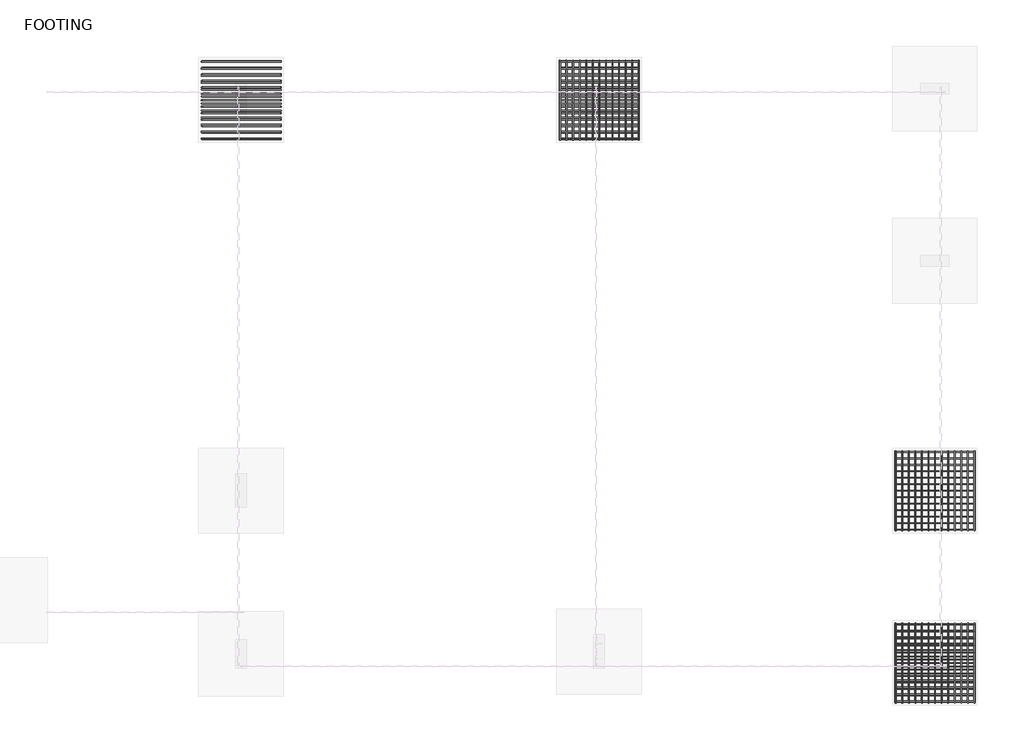
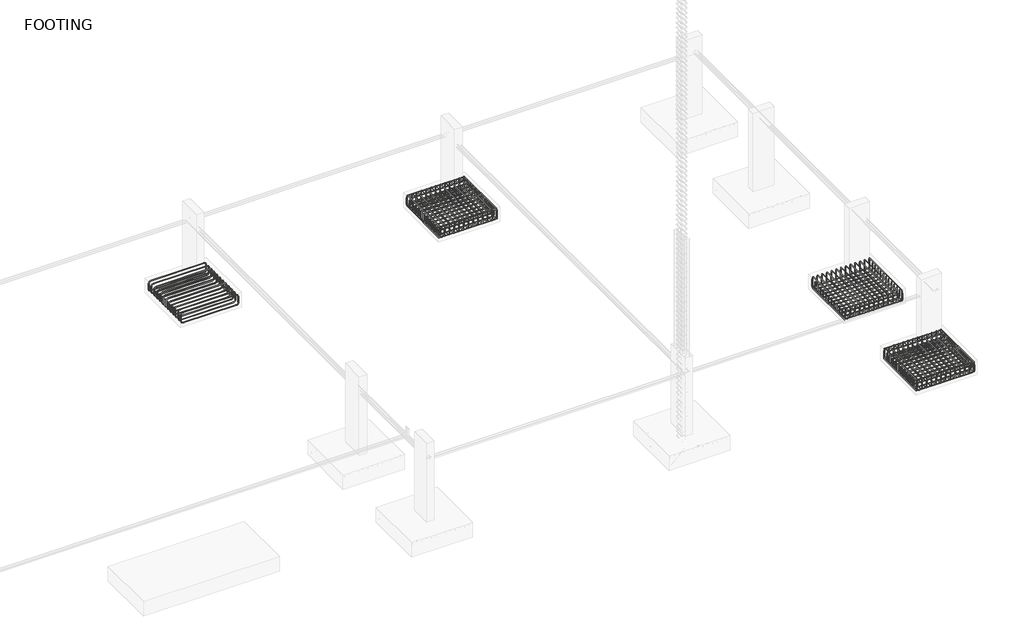
# One storey, part 8 of 12: 13 reinforcing bars.
"""IFC4 building model written with IfcOpenShell, lengths in millimetres."""

from ifc_helpers import new_model, si_unit, point, frame, origin, place, context, project, spatial, polyline, circle_curve, trimmed, segment, composite_curve, source, transform, mapped, element, save
from ifc_brep_helpers import swept_disk

model = new_model("IFC4")

# Units and contexts
model_context = context("Model", 3, world=origin())
ifc_project = project(units=[si_unit("LENGTHUNIT", "METRE", prefix="MILLI")], contexts=[model_context])

# Site, building, storey
site = spatial("IfcSite", under=ifc_project)
building = spatial("IfcBuilding", under=site)
storey = spatial("IfcBuildingStorey", under=building, Name="FOOTING", Elevation=-5638.8)

# Reinforcing bars
placement = place(None, origin())
reinforcing_bar_shape = source(origin(), model_context, "Body", "SolidModel", [
    swept_disk(composite_curve([segment(polyline([(20052.0998335, -15200.9541655, -5788.8), (20052.0998335, -15200.9541655, -5975.4)]), True, "CONTINUOUS"), segment(trimmed(circle_curve(frame((20052.0998335, -15145.5041655, -5975.4), z_axis=(1.0, 0.0, 0.0), x_axis=(0.0, -55.44999999999891, 0.0)), 55.45), [point((20052.0998335, -15200.9541655, -5975.4))], [point((20052.0998335, -15145.5041655, -6030.85))], True, "CARTESIAN"), True, "CONTINUOUS"), segment(polyline([(20052.0998335, -15145.5041655, -6030.85), (20052.0998335, -13572.3041655, -6030.85)]), True, "CONTINUOUS"), segment(trimmed(circle_curve(frame((20052.0998335, -13572.3041655, -5975.4), z_axis=(1.0, 0.0, 0.0), x_axis=(0.0, 0.0, -55.45000000000073)), 55.45), [point((20052.0998335, -13572.3041655, -6030.85))], [point((20052.0998335, -13516.8541655, -5975.4))], True, "CARTESIAN"), True, "CONTINUOUS"), segment(polyline([(20052.0998335, -13516.8541655, -5975.4), (20052.0998335, -13516.8541655, -5788.8)]), True, "CONTINUOUS")], self_intersect=False), 7.95),
])
element("IfcReinforcingBar", 1, at=placement, inside=storey, context=model_context, shape_type="MappedRepresentation", body=[
    mapped(reinforcing_bar_shape, transform((0.0, 0.0, 0.0), x_axis=(1.0, 0.0, 0.0), y_axis=(0.0, 1.0, 0.0), z_axis=(0.0, 0.0, 1.0))),
    mapped(reinforcing_bar_shape, transform((-140.3416667, 0.0, 0.0), x_axis=(1.0, 0.0, 0.0), y_axis=(0.0, 1.0, 0.0), z_axis=(0.0, 0.0, 1.0))),
    mapped(reinforcing_bar_shape, transform((-280.6833333, 0.0, 0.0), x_axis=(1.0, 0.0, 0.0), y_axis=(0.0, 1.0, 0.0), z_axis=(0.0, 0.0, 1.0))),
    mapped(reinforcing_bar_shape, transform((-421.025, 0.0, 0.0), x_axis=(1.0, 0.0, 0.0), y_axis=(0.0, 1.0, 0.0), z_axis=(0.0, 0.0, 1.0))),
    mapped(reinforcing_bar_shape, transform((-561.3666667, 0.0, 0.0), x_axis=(1.0, 0.0, 0.0), y_axis=(0.0, 1.0, 0.0), z_axis=(0.0, 0.0, 1.0))),
    mapped(reinforcing_bar_shape, transform((-701.7083333, 0.0, 0.0), x_axis=(1.0, 0.0, 0.0), y_axis=(0.0, 1.0, 0.0), z_axis=(0.0, 0.0, 1.0))),
    mapped(reinforcing_bar_shape, transform((-842.05, 0.0, 0.0), x_axis=(1.0, 0.0, 0.0), y_axis=(0.0, 1.0, 0.0), z_axis=(0.0, 0.0, 1.0))),
    mapped(reinforcing_bar_shape, transform((-982.3916667, 0.0, 0.0), x_axis=(1.0, 0.0, 0.0), y_axis=(0.0, 1.0, 0.0), z_axis=(0.0, 0.0, 1.0))),
    mapped(reinforcing_bar_shape, transform((-1122.7333333, 0.0, 0.0), x_axis=(1.0, 0.0, 0.0), y_axis=(0.0, 1.0, 0.0), z_axis=(0.0, 0.0, 1.0))),
    mapped(reinforcing_bar_shape, transform((-1263.075, 0.0, 0.0), x_axis=(1.0, 0.0, 0.0), y_axis=(0.0, 1.0, 0.0), z_axis=(0.0, 0.0, 1.0))),
    mapped(reinforcing_bar_shape, transform((-1403.4166667, 0.0, 0.0), x_axis=(1.0, 0.0, 0.0), y_axis=(0.0, 1.0, 0.0), z_axis=(0.0, 0.0, 1.0))),
    mapped(reinforcing_bar_shape, transform((-1543.7583333, 0.0, 0.0), x_axis=(1.0, 0.0, 0.0), y_axis=(0.0, 1.0, 0.0), z_axis=(0.0, 0.0, 1.0))),
    mapped(reinforcing_bar_shape, transform((-1684.1, 0.0, 0.0), x_axis=(1.0, 0.0, 0.0), y_axis=(0.0, 1.0, 0.0), z_axis=(0.0, 0.0, 1.0))),
])
reinforcing_bar_2_shape = source(origin(), model_context, "Body", "SolidModel", [
    swept_disk(composite_curve([segment(polyline([(20042.9597994, -13515.2541655, -5888.8), (20042.9597994, -13515.2541655, -5741.5)]), True, "CONTINUOUS"), segment(trimmed(circle_curve(frame((20042.9597994, -13561.6041655, -5741.5), z_axis=(1.0, 0.0, 0.0), x_axis=(0.0, 46.350000000000364, 0.0)), 46.35), [point((20042.9597994, -13515.2541655, -5741.5))], [point((20042.9597994, -13561.6041655, -5695.15))], True, "CARTESIAN"), True, "CONTINUOUS"), segment(polyline([(20042.9597994, -13561.6041655, -5695.15), (20042.9597994, -15156.2041655, -5695.15)]), True, "CONTINUOUS"), segment(trimmed(circle_curve(frame((20042.9597994, -15156.2041655, -5741.5), z_axis=(1.0, 0.0, 0.0), x_axis=(0.0, 0.0, 46.350000000000364)), 46.35), [point((20042.9597994, -15156.2041655, -5695.15))], [point((20042.9597994, -15202.5541655, -5741.5))], True, "CARTESIAN"), True, "CONTINUOUS"), segment(polyline([(20042.9597994, -15202.5541655, -5741.5), (20042.9597994, -15202.5541655, -5888.8)]), True, "CONTINUOUS")], self_intersect=False), 6.35),
])
element("IfcReinforcingBar", 2, at=placement, inside=storey, context=model_context, shape_type="MappedRepresentation", body=[
    mapped(reinforcing_bar_2_shape, transform((0.0, 0.0, 0.0), x_axis=(1.0, 0.0, 0.0), y_axis=(0.0, 1.0, 0.0), z_axis=(0.0, 0.0, 1.0))),
    mapped(reinforcing_bar_2_shape, transform((-138.4829293, 0.0, 0.0), x_axis=(1.0, 0.0, 0.0), y_axis=(0.0, 1.0, 0.0), z_axis=(0.0, 0.0, 1.0))),
    mapped(reinforcing_bar_2_shape, transform((-276.9658586, 0.0, 0.0), x_axis=(1.0, 0.0, 0.0), y_axis=(0.0, 1.0, 0.0), z_axis=(0.0, 0.0, 1.0))),
    mapped(reinforcing_bar_2_shape, transform((-415.4487879, 0.0, 0.0), x_axis=(1.0, 0.0, 0.0), y_axis=(0.0, 1.0, 0.0), z_axis=(0.0, 0.0, 1.0))),
    mapped(reinforcing_bar_2_shape, transform((-553.9317172, 0.0, 0.0), x_axis=(1.0, 0.0, 0.0), y_axis=(0.0, 1.0, 0.0), z_axis=(0.0, 0.0, 1.0))),
    mapped(reinforcing_bar_2_shape, transform((-692.4146465, 0.0, 0.0), x_axis=(1.0, 0.0, 0.0), y_axis=(0.0, 1.0, 0.0), z_axis=(0.0, 0.0, 1.0))),
    mapped(reinforcing_bar_2_shape, transform((-830.8975758, 0.0, 0.0), x_axis=(1.0, 0.0, 0.0), y_axis=(0.0, 1.0, 0.0), z_axis=(0.0, 0.0, 1.0))),
    mapped(reinforcing_bar_2_shape, transform((-969.3805051, 0.0, 0.0), x_axis=(1.0, 0.0, 0.0), y_axis=(0.0, 1.0, 0.0), z_axis=(0.0, 0.0, 1.0))),
    mapped(reinforcing_bar_2_shape, transform((-1107.8634344, 0.0, 0.0), x_axis=(1.0, 0.0, 0.0), y_axis=(0.0, 1.0, 0.0), z_axis=(0.0, 0.0, 1.0))),
    mapped(reinforcing_bar_2_shape, transform((-1246.3463637, 0.0, 0.0), x_axis=(1.0, 0.0, 0.0), y_axis=(0.0, 1.0, 0.0), z_axis=(0.0, 0.0, 1.0))),
    mapped(reinforcing_bar_2_shape, transform((-1384.8292929, 0.0, 0.0), x_axis=(1.0, 0.0, 0.0), y_axis=(0.0, 1.0, 0.0), z_axis=(0.0, 0.0, 1.0))),
    mapped(reinforcing_bar_2_shape, transform((-1523.3122222, 0.0, 0.0), x_axis=(1.0, 0.0, 0.0), y_axis=(0.0, 1.0, 0.0), z_axis=(0.0, 0.0, 1.0))),
    mapped(reinforcing_bar_2_shape, transform((-1661.7951515, 0.0, 0.0), x_axis=(1.0, 0.0, 0.0), y_axis=(0.0, 1.0, 0.0), z_axis=(0.0, 0.0, 1.0))),
])
reinforcing_bar_3_shape = source(origin(), model_context, "Body", "SolidModel", [
    swept_disk(composite_curve([segment(polyline([(18367.9998335, -15183.9041655, -5773.0), (18367.9998335, -15183.9041655, -5959.6)]), True, "CONTINUOUS"), segment(trimmed(circle_curve(frame((18423.4498335, -15183.9041655, -5959.6), z_axis=(0.0, -1.0, 0.0), x_axis=(-55.45000000000073, 0.0, 0.0)), 55.45), [point((18367.9998335, -15183.9041655, -5959.6))], [point((18423.4498335, -15183.9041655, -6015.05))], True, "CARTESIAN"), True, "CONTINUOUS"), segment(polyline([(18423.4498335, -15183.9041655, -6015.05), (19996.6498335, -15183.9041655, -6015.05)]), True, "CONTINUOUS"), segment(trimmed(circle_curve(frame((19996.6498335, -15183.9041655, -5959.6), z_axis=(0.0, -1.0, 0.0), x_axis=(0.0, 0.0, -55.44999999999982)), 55.45), [point((19996.6498335, -15183.9041655, -6015.05))], [point((20052.0998335, -15183.9041655, -5959.6))], True, "CARTESIAN"), True, "CONTINUOUS"), segment(polyline([(20052.0998335, -15183.9041655, -5959.6), (20052.0998335, -15183.9041655, -5773.0)]), True, "CONTINUOUS")], self_intersect=False), 7.95),
])
element("IfcReinforcingBar", 3, at=placement, inside=storey, context=model_context, shape_type="MappedRepresentation", body=[
    mapped(reinforcing_bar_3_shape, transform((0.0, 0.0, 0.0), x_axis=(1.0, 0.0, 0.0), y_axis=(0.0, 1.0, 0.0), z_axis=(0.0, 0.0, 1.0))),
    mapped(reinforcing_bar_3_shape, transform((0.0, 137.7402087, 0.0), x_axis=(1.0, 0.0, 0.0), y_axis=(0.0, 1.0, 0.0), z_axis=(0.0, 0.0, 1.0))),
    mapped(reinforcing_bar_3_shape, transform((0.0, 275.4804175, 0.0), x_axis=(1.0, 0.0, 0.0), y_axis=(0.0, 1.0, 0.0), z_axis=(0.0, 0.0, 1.0))),
    mapped(reinforcing_bar_3_shape, transform((0.0, 413.2206262, 0.0), x_axis=(1.0, 0.0, 0.0), y_axis=(0.0, 1.0, 0.0), z_axis=(0.0, 0.0, 1.0))),
    mapped(reinforcing_bar_3_shape, transform((0.0, 550.960835, 0.0), x_axis=(1.0, 0.0, 0.0), y_axis=(0.0, 1.0, 0.0), z_axis=(0.0, 0.0, 1.0))),
    mapped(reinforcing_bar_3_shape, transform((0.0, 688.7010437, 0.0), x_axis=(1.0, 0.0, 0.0), y_axis=(0.0, 1.0, 0.0), z_axis=(0.0, 0.0, 1.0))),
    mapped(reinforcing_bar_3_shape, transform((0.0, 826.4412525, 0.0), x_axis=(1.0, 0.0, 0.0), y_axis=(0.0, 1.0, 0.0), z_axis=(0.0, 0.0, 1.0))),
    mapped(reinforcing_bar_3_shape, transform((0.0, 964.1814612, 0.0), x_axis=(1.0, 0.0, 0.0), y_axis=(0.0, 1.0, 0.0), z_axis=(0.0, 0.0, 1.0))),
    mapped(reinforcing_bar_3_shape, transform((0.0, 1101.92167, 0.0), x_axis=(1.0, 0.0, 0.0), y_axis=(0.0, 1.0, 0.0), z_axis=(0.0, 0.0, 1.0))),
    mapped(reinforcing_bar_3_shape, transform((0.0, 1239.6618787, 0.0), x_axis=(1.0, 0.0, 0.0), y_axis=(0.0, 1.0, 0.0), z_axis=(0.0, 0.0, 1.0))),
    mapped(reinforcing_bar_3_shape, transform((0.0, 1377.4020875, 0.0), x_axis=(1.0, 0.0, 0.0), y_axis=(0.0, 1.0, 0.0), z_axis=(0.0, 0.0, 1.0))),
    mapped(reinforcing_bar_3_shape, transform((0.0, 1515.1422962, 0.0), x_axis=(1.0, 0.0, 0.0), y_axis=(0.0, 1.0, 0.0), z_axis=(0.0, 0.0, 1.0))),
    mapped(reinforcing_bar_3_shape, transform((0.0, 1652.882505, 0.0), x_axis=(1.0, 0.0, 0.0), y_axis=(0.0, 1.0, 0.0), z_axis=(0.0, 0.0, 1.0))),
])
reinforcing_bar_4_shape = source(origin(), model_context, "Body", "SolidModel", [
    swept_disk(composite_curve([segment(polyline([(18367.9998335, -13541.2399866, -5950.85), (18367.9998335, -13541.2399866, -5764.25)]), True, "CONTINUOUS"), segment(trimmed(circle_curve(frame((18423.4498335, -13541.2399866, -5764.25), z_axis=(0.0, 1.0, 0.0), x_axis=(-55.45000000000073, 0.0, 0.0)), 55.45), [point((18367.9998335, -13541.2399866, -5764.25))], [point((18423.4498335, -13541.2399866, -5708.8))], True, "CARTESIAN"), True, "CONTINUOUS"), segment(polyline([(18423.4498335, -13541.2399866, -5708.8), (19996.6498335, -13541.2399866, -5708.8)]), True, "CONTINUOUS"), segment(trimmed(circle_curve(frame((19996.6498335, -13541.2399866, -5764.25), z_axis=(0.0, 1.0, 0.0), x_axis=(0.0, 0.0, 55.44999999999982)), 55.45), [point((19996.6498335, -13541.2399866, -5708.8))], [point((20052.0998335, -13541.2399866, -5764.25))], True, "CARTESIAN"), True, "CONTINUOUS"), segment(polyline([(20052.0998335, -13541.2399866, -5764.25), (20052.0998335, -13541.2399866, -5950.85)]), True, "CONTINUOUS")], self_intersect=False), 7.95),
])
element("IfcReinforcingBar", 4, at=placement, inside=storey, context=model_context, shape_type="MappedRepresentation", body=[
    mapped(reinforcing_bar_4_shape, transform((0.0, 0.0, 0.0), x_axis=(1.0, 0.0, 0.0), y_axis=(0.0, 1.0, 0.0), z_axis=(0.0, 0.0, 1.0))),
    mapped(reinforcing_bar_4_shape, transform((0.0, -148.1882348, 0.0), x_axis=(1.0, 0.0, 0.0), y_axis=(0.0, 1.0, 0.0), z_axis=(0.0, 0.0, 1.0))),
    mapped(reinforcing_bar_4_shape, transform((0.0, -296.3764695, 0.0), x_axis=(1.0, 0.0, 0.0), y_axis=(0.0, 1.0, 0.0), z_axis=(0.0, 0.0, 1.0))),
    mapped(reinforcing_bar_4_shape, transform((0.0, -444.5647043, 0.0), x_axis=(1.0, 0.0, 0.0), y_axis=(0.0, 1.0, 0.0), z_axis=(0.0, 0.0, 1.0))),
    mapped(reinforcing_bar_4_shape, transform((0.0, -592.7529391, 0.0), x_axis=(1.0, 0.0, 0.0), y_axis=(0.0, 1.0, 0.0), z_axis=(0.0, 0.0, 1.0))),
    mapped(reinforcing_bar_4_shape, transform((0.0, -740.9411738, 0.0), x_axis=(1.0, 0.0, 0.0), y_axis=(0.0, 1.0, 0.0), z_axis=(0.0, 0.0, 1.0))),
    mapped(reinforcing_bar_4_shape, transform((0.0, -889.1294086, 0.0), x_axis=(1.0, 0.0, 0.0), y_axis=(0.0, 1.0, 0.0), z_axis=(0.0, 0.0, 1.0))),
    mapped(reinforcing_bar_4_shape, transform((0.0, -1037.3176434, 0.0), x_axis=(1.0, 0.0, 0.0), y_axis=(0.0, 1.0, 0.0), z_axis=(0.0, 0.0, 1.0))),
    mapped(reinforcing_bar_4_shape, transform((0.0, -1185.5058782, 0.0), x_axis=(1.0, 0.0, 0.0), y_axis=(0.0, 1.0, 0.0), z_axis=(0.0, 0.0, 1.0))),
    mapped(reinforcing_bar_4_shape, transform((0.0, -1333.6941129, 0.0), x_axis=(1.0, 0.0, 0.0), y_axis=(0.0, 1.0, 0.0), z_axis=(0.0, 0.0, 1.0))),
    mapped(reinforcing_bar_4_shape, transform((0.0, -1481.8823477, 0.0), x_axis=(1.0, 0.0, 0.0), y_axis=(0.0, 1.0, 0.0), z_axis=(0.0, 0.0, 1.0))),
    mapped(reinforcing_bar_4_shape, transform((0.0, -1630.0705825, 0.0), x_axis=(1.0, 0.0, 0.0), y_axis=(0.0, 1.0, 0.0), z_axis=(0.0, 0.0, 1.0))),
])
reinforcing_bar_5_shape = source(origin(), model_context, "Body", "SolidModel", [
    swept_disk(composite_curve([segment(polyline([(20052.0998335, -11543.3541655, -5788.8), (20052.0998335, -11543.3541655, -5975.4)]), True, "CONTINUOUS"), segment(trimmed(circle_curve(frame((20052.0998335, -11487.9041655, -5975.4), z_axis=(1.0, 0.0, 0.0), x_axis=(0.0, -55.45000000000073, 0.0)), 55.45), [point((20052.0998335, -11543.3541655, -5975.4))], [point((20052.0998335, -11487.9041655, -6030.85))], True, "CARTESIAN"), True, "CONTINUOUS"), segment(polyline([(20052.0998335, -11487.9041655, -6030.85), (20052.0998335, -9914.7041655, -6030.85)]), True, "CONTINUOUS"), segment(trimmed(circle_curve(frame((20052.0998335, -9914.7041655, -5975.4), z_axis=(1.0, 0.0, 0.0), x_axis=(0.0, 0.0, -55.45000000000073)), 55.45), [point((20052.0998335, -9914.7041655, -6030.85))], [point((20052.0998335, -9859.2541655, -5975.4))], True, "CARTESIAN"), True, "CONTINUOUS"), segment(polyline([(20052.0998335, -9859.2541655, -5975.4), (20052.0998335, -9859.2541655, -5788.8)]), True, "CONTINUOUS")], self_intersect=False), 7.95),
])
element("IfcReinforcingBar", 5, at=placement, inside=storey, context=model_context, shape_type="MappedRepresentation", body=[
    mapped(reinforcing_bar_5_shape, transform((0.0, 0.0, 0.0), x_axis=(1.0, 0.0, 0.0), y_axis=(0.0, 1.0, 0.0), z_axis=(0.0, 0.0, 1.0))),
    mapped(reinforcing_bar_5_shape, transform((-140.3416667, 0.0, 0.0), x_axis=(1.0, 0.0, 0.0), y_axis=(0.0, 1.0, 0.0), z_axis=(0.0, 0.0, 1.0))),
    mapped(reinforcing_bar_5_shape, transform((-280.6833333, 0.0, 0.0), x_axis=(1.0, 0.0, 0.0), y_axis=(0.0, 1.0, 0.0), z_axis=(0.0, 0.0, 1.0))),
    mapped(reinforcing_bar_5_shape, transform((-421.025, 0.0, 0.0), x_axis=(1.0, 0.0, 0.0), y_axis=(0.0, 1.0, 0.0), z_axis=(0.0, 0.0, 1.0))),
    mapped(reinforcing_bar_5_shape, transform((-561.3666667, 0.0, 0.0), x_axis=(1.0, 0.0, 0.0), y_axis=(0.0, 1.0, 0.0), z_axis=(0.0, 0.0, 1.0))),
    mapped(reinforcing_bar_5_shape, transform((-701.7083333, 0.0, 0.0), x_axis=(1.0, 0.0, 0.0), y_axis=(0.0, 1.0, 0.0), z_axis=(0.0, 0.0, 1.0))),
    mapped(reinforcing_bar_5_shape, transform((-842.05, 0.0, 0.0), x_axis=(1.0, 0.0, 0.0), y_axis=(0.0, 1.0, 0.0), z_axis=(0.0, 0.0, 1.0))),
    mapped(reinforcing_bar_5_shape, transform((-982.3916667, 0.0, 0.0), x_axis=(1.0, 0.0, 0.0), y_axis=(0.0, 1.0, 0.0), z_axis=(0.0, 0.0, 1.0))),
    mapped(reinforcing_bar_5_shape, transform((-1122.7333333, 0.0, 0.0), x_axis=(1.0, 0.0, 0.0), y_axis=(0.0, 1.0, 0.0), z_axis=(0.0, 0.0, 1.0))),
    mapped(reinforcing_bar_5_shape, transform((-1263.075, 0.0, 0.0), x_axis=(1.0, 0.0, 0.0), y_axis=(0.0, 1.0, 0.0), z_axis=(0.0, 0.0, 1.0))),
    mapped(reinforcing_bar_5_shape, transform((-1403.4166667, 0.0, 0.0), x_axis=(1.0, 0.0, 0.0), y_axis=(0.0, 1.0, 0.0), z_axis=(0.0, 0.0, 1.0))),
    mapped(reinforcing_bar_5_shape, transform((-1543.7583333, 0.0, 0.0), x_axis=(1.0, 0.0, 0.0), y_axis=(0.0, 1.0, 0.0), z_axis=(0.0, 0.0, 1.0))),
    mapped(reinforcing_bar_5_shape, transform((-1684.1, 0.0, 0.0), x_axis=(1.0, 0.0, 0.0), y_axis=(0.0, 1.0, 0.0), z_axis=(0.0, 0.0, 1.0))),
])
reinforcing_bar_6_shape = source(origin(), model_context, "Body", "SolidModel", [
    swept_disk(composite_curve([segment(polyline([(20042.9597994, -9857.6541655, -5888.8), (20042.9597994, -9857.6541655, -5741.5)]), True, "CONTINUOUS"), segment(trimmed(circle_curve(frame((20042.9597994, -9904.0041655, -5741.5), z_axis=(1.0, 0.0, 0.0), x_axis=(0.0, 46.350000000000364, 0.0)), 46.35), [point((20042.9597994, -9857.6541655, -5741.5))], [point((20042.9597994, -9904.0041655, -5695.15))], True, "CARTESIAN"), True, "CONTINUOUS"), segment(polyline([(20042.9597994, -9904.0041655, -5695.15), (20042.9597994, -11498.6041655, -5695.15)]), True, "CONTINUOUS"), segment(trimmed(circle_curve(frame((20042.9597994, -11498.6041655, -5741.5), z_axis=(1.0, 0.0, 0.0), x_axis=(0.0, 0.0, 46.350000000000364)), 46.35), [point((20042.9597994, -11498.6041655, -5695.15))], [point((20042.9597994, -11544.9541655, -5741.5))], True, "CARTESIAN"), True, "CONTINUOUS"), segment(polyline([(20042.9597994, -11544.9541655, -5741.5), (20042.9597994, -11544.9541655, -5888.8)]), True, "CONTINUOUS")], self_intersect=False), 6.35),
])
element("IfcReinforcingBar", 6, at=placement, inside=storey, context=model_context, shape_type="MappedRepresentation", body=[
    mapped(reinforcing_bar_6_shape, transform((0.0, 0.0, 0.0), x_axis=(1.0, 0.0, 0.0), y_axis=(0.0, 1.0, 0.0), z_axis=(0.0, 0.0, 1.0))),
    mapped(reinforcing_bar_6_shape, transform((-138.4829293, 0.0, 0.0), x_axis=(1.0, 0.0, 0.0), y_axis=(0.0, 1.0, 0.0), z_axis=(0.0, 0.0, 1.0))),
    mapped(reinforcing_bar_6_shape, transform((-276.9658586, 0.0, 0.0), x_axis=(1.0, 0.0, 0.0), y_axis=(0.0, 1.0, 0.0), z_axis=(0.0, 0.0, 1.0))),
    mapped(reinforcing_bar_6_shape, transform((-415.4487879, 0.0, 0.0), x_axis=(1.0, 0.0, 0.0), y_axis=(0.0, 1.0, 0.0), z_axis=(0.0, 0.0, 1.0))),
    mapped(reinforcing_bar_6_shape, transform((-553.9317172, 0.0, 0.0), x_axis=(1.0, 0.0, 0.0), y_axis=(0.0, 1.0, 0.0), z_axis=(0.0, 0.0, 1.0))),
    mapped(reinforcing_bar_6_shape, transform((-692.4146465, 0.0, 0.0), x_axis=(1.0, 0.0, 0.0), y_axis=(0.0, 1.0, 0.0), z_axis=(0.0, 0.0, 1.0))),
    mapped(reinforcing_bar_6_shape, transform((-830.8975758, 0.0, 0.0), x_axis=(1.0, 0.0, 0.0), y_axis=(0.0, 1.0, 0.0), z_axis=(0.0, 0.0, 1.0))),
    mapped(reinforcing_bar_6_shape, transform((-969.3805051, 0.0, 0.0), x_axis=(1.0, 0.0, 0.0), y_axis=(0.0, 1.0, 0.0), z_axis=(0.0, 0.0, 1.0))),
    mapped(reinforcing_bar_6_shape, transform((-1107.8634344, 0.0, 0.0), x_axis=(1.0, 0.0, 0.0), y_axis=(0.0, 1.0, 0.0), z_axis=(0.0, 0.0, 1.0))),
    mapped(reinforcing_bar_6_shape, transform((-1246.3463637, 0.0, 0.0), x_axis=(1.0, 0.0, 0.0), y_axis=(0.0, 1.0, 0.0), z_axis=(0.0, 0.0, 1.0))),
    mapped(reinforcing_bar_6_shape, transform((-1384.8292929, 0.0, 0.0), x_axis=(1.0, 0.0, 0.0), y_axis=(0.0, 1.0, 0.0), z_axis=(0.0, 0.0, 1.0))),
    mapped(reinforcing_bar_6_shape, transform((-1523.3122222, 0.0, 0.0), x_axis=(1.0, 0.0, 0.0), y_axis=(0.0, 1.0, 0.0), z_axis=(0.0, 0.0, 1.0))),
    mapped(reinforcing_bar_6_shape, transform((-1661.7951515, 0.0, 0.0), x_axis=(1.0, 0.0, 0.0), y_axis=(0.0, 1.0, 0.0), z_axis=(0.0, 0.0, 1.0))),
])
reinforcing_bar_7_shape = source(origin(), model_context, "Body", "SolidModel", [
    swept_disk(composite_curve([segment(polyline([(18367.9998335, -11526.3041655, -5773.0), (18367.9998335, -11526.3041655, -5959.6)]), True, "CONTINUOUS"), segment(trimmed(circle_curve(frame((18423.4498335, -11526.3041655, -5959.6), z_axis=(0.0, -1.0, 0.0), x_axis=(-55.45000000000073, 0.0, 0.0)), 55.45), [point((18367.9998335, -11526.3041655, -5959.6))], [point((18423.4498335, -11526.3041655, -6015.05))], True, "CARTESIAN"), True, "CONTINUOUS"), segment(polyline([(18423.4498335, -11526.3041655, -6015.05), (19996.6498335, -11526.3041655, -6015.05)]), True, "CONTINUOUS"), segment(trimmed(circle_curve(frame((19996.6498335, -11526.3041655, -5959.6), z_axis=(0.0, -1.0, 0.0), x_axis=(0.0, 0.0, -55.44999999999982)), 55.45), [point((19996.6498335, -11526.3041655, -6015.05))], [point((20052.0998335, -11526.3041655, -5959.6))], True, "CARTESIAN"), True, "CONTINUOUS"), segment(polyline([(20052.0998335, -11526.3041655, -5959.6), (20052.0998335, -11526.3041655, -5773.0)]), True, "CONTINUOUS")], self_intersect=False), 7.95),
])
element("IfcReinforcingBar", 7, at=placement, inside=storey, context=model_context, shape_type="MappedRepresentation", body=[
    mapped(reinforcing_bar_7_shape, transform((0.0, 0.0, 0.0), x_axis=(1.0, 0.0, 0.0), y_axis=(0.0, 1.0, 0.0), z_axis=(0.0, 0.0, 1.0))),
    mapped(reinforcing_bar_7_shape, transform((0.0, 137.7402087, 0.0), x_axis=(1.0, 0.0, 0.0), y_axis=(0.0, 1.0, 0.0), z_axis=(0.0, 0.0, 1.0))),
    mapped(reinforcing_bar_7_shape, transform((0.0, 275.4804175, 0.0), x_axis=(1.0, 0.0, 0.0), y_axis=(0.0, 1.0, 0.0), z_axis=(0.0, 0.0, 1.0))),
    mapped(reinforcing_bar_7_shape, transform((0.0, 413.2206262, 0.0), x_axis=(1.0, 0.0, 0.0), y_axis=(0.0, 1.0, 0.0), z_axis=(0.0, 0.0, 1.0))),
    mapped(reinforcing_bar_7_shape, transform((0.0, 550.960835, 0.0), x_axis=(1.0, 0.0, 0.0), y_axis=(0.0, 1.0, 0.0), z_axis=(0.0, 0.0, 1.0))),
    mapped(reinforcing_bar_7_shape, transform((0.0, 688.7010437, 0.0), x_axis=(1.0, 0.0, 0.0), y_axis=(0.0, 1.0, 0.0), z_axis=(0.0, 0.0, 1.0))),
    mapped(reinforcing_bar_7_shape, transform((0.0, 826.4412525, 0.0), x_axis=(1.0, 0.0, 0.0), y_axis=(0.0, 1.0, 0.0), z_axis=(0.0, 0.0, 1.0))),
    mapped(reinforcing_bar_7_shape, transform((0.0, 964.1814612, 0.0), x_axis=(1.0, 0.0, 0.0), y_axis=(0.0, 1.0, 0.0), z_axis=(0.0, 0.0, 1.0))),
    mapped(reinforcing_bar_7_shape, transform((0.0, 1101.92167, 0.0), x_axis=(1.0, 0.0, 0.0), y_axis=(0.0, 1.0, 0.0), z_axis=(0.0, 0.0, 1.0))),
    mapped(reinforcing_bar_7_shape, transform((0.0, 1239.6618787, 0.0), x_axis=(1.0, 0.0, 0.0), y_axis=(0.0, 1.0, 0.0), z_axis=(0.0, 0.0, 1.0))),
    mapped(reinforcing_bar_7_shape, transform((0.0, 1377.4020875, 0.0), x_axis=(1.0, 0.0, 0.0), y_axis=(0.0, 1.0, 0.0), z_axis=(0.0, 0.0, 1.0))),
    mapped(reinforcing_bar_7_shape, transform((0.0, 1515.1422962, 0.0), x_axis=(1.0, 0.0, 0.0), y_axis=(0.0, 1.0, 0.0), z_axis=(0.0, 0.0, 1.0))),
    mapped(reinforcing_bar_7_shape, transform((0.0, 1652.882505, 0.0), x_axis=(1.0, 0.0, 0.0), y_axis=(0.0, 1.0, 0.0), z_axis=(0.0, 0.0, 1.0))),
])
reinforcing_bar_8_shape = source(origin(), model_context, "Body", "SolidModel", [
    swept_disk(composite_curve([segment(polyline([(12927.3998335, -3250.2541655, -5788.8), (12927.3998335, -3250.2541655, -5975.4)]), True, "CONTINUOUS"), segment(trimmed(circle_curve(frame((12927.3998335, -3194.8041655, -5975.4), z_axis=(1.0, 0.0, 0.0), x_axis=(0.0, -55.44999999999982, 0.0)), 55.45), [point((12927.3998335, -3250.2541655, -5975.4))], [point((12927.3998335, -3194.8041655, -6030.85))], True, "CARTESIAN"), True, "CONTINUOUS"), segment(polyline([(12927.3998335, -3194.8041655, -6030.85), (12927.3998335, -1621.6041655, -6030.85)]), True, "CONTINUOUS"), segment(trimmed(circle_curve(frame((12927.3998335, -1621.6041655, -5975.4), z_axis=(1.0, 0.0, 0.0), x_axis=(0.0, 0.0, -55.45000000000073)), 55.45), [point((12927.3998335, -1621.6041655, -6030.85))], [point((12927.3998335, -1566.1541655, -5975.4))], True, "CARTESIAN"), True, "CONTINUOUS"), segment(polyline([(12927.3998335, -1566.1541655, -5975.4), (12927.3998335, -1566.1541655, -5788.8)]), True, "CONTINUOUS")], self_intersect=False), 7.95),
])
element("IfcReinforcingBar", 8, at=placement, inside=storey, context=model_context, shape_type="MappedRepresentation", body=[
    mapped(reinforcing_bar_8_shape, transform((0.0, 0.0, 0.0), x_axis=(1.0, 0.0, 0.0), y_axis=(0.0, 1.0, 0.0), z_axis=(0.0, 0.0, 1.0))),
    mapped(reinforcing_bar_8_shape, transform((-140.3416667, 0.0, 0.0), x_axis=(1.0, 0.0, 0.0), y_axis=(0.0, 1.0, 0.0), z_axis=(0.0, 0.0, 1.0))),
    mapped(reinforcing_bar_8_shape, transform((-280.6833333, 0.0, 0.0), x_axis=(1.0, 0.0, 0.0), y_axis=(0.0, 1.0, 0.0), z_axis=(0.0, 0.0, 1.0))),
    mapped(reinforcing_bar_8_shape, transform((-421.025, 0.0, 0.0), x_axis=(1.0, 0.0, 0.0), y_axis=(0.0, 1.0, 0.0), z_axis=(0.0, 0.0, 1.0))),
    mapped(reinforcing_bar_8_shape, transform((-561.3666667, 0.0, 0.0), x_axis=(1.0, 0.0, 0.0), y_axis=(0.0, 1.0, 0.0), z_axis=(0.0, 0.0, 1.0))),
    mapped(reinforcing_bar_8_shape, transform((-701.7083333, 0.0, 0.0), x_axis=(1.0, 0.0, 0.0), y_axis=(0.0, 1.0, 0.0), z_axis=(0.0, 0.0, 1.0))),
    mapped(reinforcing_bar_8_shape, transform((-842.05, 0.0, 0.0), x_axis=(1.0, 0.0, 0.0), y_axis=(0.0, 1.0, 0.0), z_axis=(0.0, 0.0, 1.0))),
    mapped(reinforcing_bar_8_shape, transform((-982.3916667, 0.0, 0.0), x_axis=(1.0, 0.0, 0.0), y_axis=(0.0, 1.0, 0.0), z_axis=(0.0, 0.0, 1.0))),
    mapped(reinforcing_bar_8_shape, transform((-1122.7333333, 0.0, 0.0), x_axis=(1.0, 0.0, 0.0), y_axis=(0.0, 1.0, 0.0), z_axis=(0.0, 0.0, 1.0))),
    mapped(reinforcing_bar_8_shape, transform((-1263.075, 0.0, 0.0), x_axis=(1.0, 0.0, 0.0), y_axis=(0.0, 1.0, 0.0), z_axis=(0.0, 0.0, 1.0))),
    mapped(reinforcing_bar_8_shape, transform((-1403.4166667, 0.0, 0.0), x_axis=(1.0, 0.0, 0.0), y_axis=(0.0, 1.0, 0.0), z_axis=(0.0, 0.0, 1.0))),
    mapped(reinforcing_bar_8_shape, transform((-1543.7583333, 0.0, 0.0), x_axis=(1.0, 0.0, 0.0), y_axis=(0.0, 1.0, 0.0), z_axis=(0.0, 0.0, 1.0))),
    mapped(reinforcing_bar_8_shape, transform((-1684.1, 0.0, 0.0), x_axis=(1.0, 0.0, 0.0), y_axis=(0.0, 1.0, 0.0), z_axis=(0.0, 0.0, 1.0))),
])
reinforcing_bar_9_shape = source(origin(), model_context, "Body", "SolidModel", [
    swept_disk(composite_curve([segment(polyline([(12918.2597994, -1564.5541655, -5888.8), (12918.2597994, -1564.5541655, -5741.5)]), True, "CONTINUOUS"), segment(trimmed(circle_curve(frame((12918.2597994, -1610.9041655, -5741.5), z_axis=(1.0, 0.0, 0.0), x_axis=(0.0, 46.350000000000136, 0.0)), 46.35), [point((12918.2597994, -1564.5541655, -5741.5))], [point((12918.2597994, -1610.9041655, -5695.15))], True, "CARTESIAN"), True, "CONTINUOUS"), segment(polyline([(12918.2597994, -1610.9041655, -5695.15), (12918.2597994, -3205.5041655, -5695.15)]), True, "CONTINUOUS"), segment(trimmed(circle_curve(frame((12918.2597994, -3205.5041655, -5741.5), z_axis=(1.0, 0.0, 0.0), x_axis=(0.0, 0.0, 46.350000000000364)), 46.35), [point((12918.2597994, -3205.5041655, -5695.15))], [point((12918.2597994, -3251.8541655, -5741.5))], True, "CARTESIAN"), True, "CONTINUOUS"), segment(polyline([(12918.2597994, -3251.8541655, -5741.5), (12918.2597994, -3251.8541655, -5888.8)]), True, "CONTINUOUS")], self_intersect=False), 6.35),
])
element("IfcReinforcingBar", 9, at=placement, inside=storey, context=model_context, shape_type="MappedRepresentation", body=[
    mapped(reinforcing_bar_9_shape, transform((0.0, 0.0, 0.0), x_axis=(1.0, 0.0, 0.0), y_axis=(0.0, 1.0, 0.0), z_axis=(0.0, 0.0, 1.0))),
    mapped(reinforcing_bar_9_shape, transform((-138.4829293, 0.0, 0.0), x_axis=(1.0, 0.0, 0.0), y_axis=(0.0, 1.0, 0.0), z_axis=(0.0, 0.0, 1.0))),
    mapped(reinforcing_bar_9_shape, transform((-276.9658586, 0.0, 0.0), x_axis=(1.0, 0.0, 0.0), y_axis=(0.0, 1.0, 0.0), z_axis=(0.0, 0.0, 1.0))),
    mapped(reinforcing_bar_9_shape, transform((-415.4487879, 0.0, 0.0), x_axis=(1.0, 0.0, 0.0), y_axis=(0.0, 1.0, 0.0), z_axis=(0.0, 0.0, 1.0))),
    mapped(reinforcing_bar_9_shape, transform((-553.9317172, 0.0, 0.0), x_axis=(1.0, 0.0, 0.0), y_axis=(0.0, 1.0, 0.0), z_axis=(0.0, 0.0, 1.0))),
    mapped(reinforcing_bar_9_shape, transform((-692.4146465, 0.0, 0.0), x_axis=(1.0, 0.0, 0.0), y_axis=(0.0, 1.0, 0.0), z_axis=(0.0, 0.0, 1.0))),
    mapped(reinforcing_bar_9_shape, transform((-830.8975758, 0.0, 0.0), x_axis=(1.0, 0.0, 0.0), y_axis=(0.0, 1.0, 0.0), z_axis=(0.0, 0.0, 1.0))),
    mapped(reinforcing_bar_9_shape, transform((-969.3805051, 0.0, 0.0), x_axis=(1.0, 0.0, 0.0), y_axis=(0.0, 1.0, 0.0), z_axis=(0.0, 0.0, 1.0))),
    mapped(reinforcing_bar_9_shape, transform((-1107.8634344, 0.0, 0.0), x_axis=(1.0, 0.0, 0.0), y_axis=(0.0, 1.0, 0.0), z_axis=(0.0, 0.0, 1.0))),
    mapped(reinforcing_bar_9_shape, transform((-1246.3463637, 0.0, 0.0), x_axis=(1.0, 0.0, 0.0), y_axis=(0.0, 1.0, 0.0), z_axis=(0.0, 0.0, 1.0))),
    mapped(reinforcing_bar_9_shape, transform((-1384.8292929, 0.0, 0.0), x_axis=(1.0, 0.0, 0.0), y_axis=(0.0, 1.0, 0.0), z_axis=(0.0, 0.0, 1.0))),
    mapped(reinforcing_bar_9_shape, transform((-1523.3122222, 0.0, 0.0), x_axis=(1.0, 0.0, 0.0), y_axis=(0.0, 1.0, 0.0), z_axis=(0.0, 0.0, 1.0))),
    mapped(reinforcing_bar_9_shape, transform((-1661.7951515, 0.0, 0.0), x_axis=(1.0, 0.0, 0.0), y_axis=(0.0, 1.0, 0.0), z_axis=(0.0, 0.0, 1.0))),
])
reinforcing_bar_10_shape = source(origin(), model_context, "Body", "SolidModel", [
    swept_disk(composite_curve([segment(polyline([(11243.2998335, -3233.2041655, -5773.0), (11243.2998335, -3233.2041655, -5959.6)]), True, "CONTINUOUS"), segment(trimmed(circle_curve(frame((11298.7498335, -3233.2041655, -5959.6), z_axis=(0.0, -1.0, 0.0), x_axis=(-55.45000000000073, 0.0, 0.0)), 55.45), [point((11243.2998335, -3233.2041655, -5959.6))], [point((11298.7498335, -3233.2041655, -6015.05))], True, "CARTESIAN"), True, "CONTINUOUS"), segment(polyline([(11298.7498335, -3233.2041655, -6015.05), (12871.9498335, -3233.2041655, -6015.05)]), True, "CONTINUOUS"), segment(trimmed(circle_curve(frame((12871.9498335, -3233.2041655, -5959.6), z_axis=(0.0, -1.0, 0.0), x_axis=(0.0, 0.0, -55.44999999999982)), 55.45), [point((12871.9498335, -3233.2041655, -6015.05))], [point((12927.3998335, -3233.2041655, -5959.6))], True, "CARTESIAN"), True, "CONTINUOUS"), segment(polyline([(12927.3998335, -3233.2041655, -5959.6), (12927.3998335, -3233.2041655, -5773.0)]), True, "CONTINUOUS")], self_intersect=False), 7.95),
])
element("IfcReinforcingBar", 10, at=placement, inside=storey, context=model_context, shape_type="MappedRepresentation", body=[
    mapped(reinforcing_bar_10_shape, transform((0.0, 0.0, 0.0), x_axis=(1.0, 0.0, 0.0), y_axis=(0.0, 1.0, 0.0), z_axis=(0.0, 0.0, 1.0))),
    mapped(reinforcing_bar_10_shape, transform((0.0, 137.7402087, 0.0), x_axis=(1.0, 0.0, 0.0), y_axis=(0.0, 1.0, 0.0), z_axis=(0.0, 0.0, 1.0))),
    mapped(reinforcing_bar_10_shape, transform((0.0, 275.4804175, 0.0), x_axis=(1.0, 0.0, 0.0), y_axis=(0.0, 1.0, 0.0), z_axis=(0.0, 0.0, 1.0))),
    mapped(reinforcing_bar_10_shape, transform((0.0, 413.2206262, 0.0), x_axis=(1.0, 0.0, 0.0), y_axis=(0.0, 1.0, 0.0), z_axis=(0.0, 0.0, 1.0))),
    mapped(reinforcing_bar_10_shape, transform((0.0, 550.960835, 0.0), x_axis=(1.0, 0.0, 0.0), y_axis=(0.0, 1.0, 0.0), z_axis=(0.0, 0.0, 1.0))),
    mapped(reinforcing_bar_10_shape, transform((0.0, 688.7010437, 0.0), x_axis=(1.0, 0.0, 0.0), y_axis=(0.0, 1.0, 0.0), z_axis=(0.0, 0.0, 1.0))),
    mapped(reinforcing_bar_10_shape, transform((0.0, 826.4412525, 0.0), x_axis=(1.0, 0.0, 0.0), y_axis=(0.0, 1.0, 0.0), z_axis=(0.0, 0.0, 1.0))),
    mapped(reinforcing_bar_10_shape, transform((0.0, 964.1814612, 0.0), x_axis=(1.0, 0.0, 0.0), y_axis=(0.0, 1.0, 0.0), z_axis=(0.0, 0.0, 1.0))),
    mapped(reinforcing_bar_10_shape, transform((0.0, 1101.92167, 0.0), x_axis=(1.0, 0.0, 0.0), y_axis=(0.0, 1.0, 0.0), z_axis=(0.0, 0.0, 1.0))),
    mapped(reinforcing_bar_10_shape, transform((0.0, 1239.6618787, 0.0), x_axis=(1.0, 0.0, 0.0), y_axis=(0.0, 1.0, 0.0), z_axis=(0.0, 0.0, 1.0))),
    mapped(reinforcing_bar_10_shape, transform((0.0, 1377.4020875, 0.0), x_axis=(1.0, 0.0, 0.0), y_axis=(0.0, 1.0, 0.0), z_axis=(0.0, 0.0, 1.0))),
    mapped(reinforcing_bar_10_shape, transform((0.0, 1515.1422962, 0.0), x_axis=(1.0, 0.0, 0.0), y_axis=(0.0, 1.0, 0.0), z_axis=(0.0, 0.0, 1.0))),
    mapped(reinforcing_bar_10_shape, transform((0.0, 1652.882505, 0.0), x_axis=(1.0, 0.0, 0.0), y_axis=(0.0, 1.0, 0.0), z_axis=(0.0, 0.0, 1.0))),
])
reinforcing_bar_11_shape = source(origin(), model_context, "Body", "SolidModel", [
    swept_disk(composite_curve([segment(polyline([(11243.2998335, -1590.5399866, -5950.85), (11243.2998335, -1590.5399866, -5764.25)]), True, "CONTINUOUS"), segment(trimmed(circle_curve(frame((11298.7498335, -1590.5399866, -5764.25), z_axis=(0.0, 1.0, 0.0), x_axis=(-55.45000000000073, 0.0, 0.0)), 55.45), [point((11243.2998335, -1590.5399866, -5764.25))], [point((11298.7498335, -1590.5399866, -5708.8))], True, "CARTESIAN"), True, "CONTINUOUS"), segment(polyline([(11298.7498335, -1590.5399866, -5708.8), (12871.9498335, -1590.5399866, -5708.8)]), True, "CONTINUOUS"), segment(trimmed(circle_curve(frame((12871.9498335, -1590.5399866, -5764.25), z_axis=(0.0, 1.0, 0.0), x_axis=(0.0, 0.0, 55.44999999999982)), 55.45), [point((12871.9498335, -1590.5399866, -5708.8))], [point((12927.3998335, -1590.5399866, -5764.25))], True, "CARTESIAN"), True, "CONTINUOUS"), segment(polyline([(12927.3998335, -1590.5399866, -5764.25), (12927.3998335, -1590.5399866, -5950.85)]), True, "CONTINUOUS")], self_intersect=False), 7.95),
])
element("IfcReinforcingBar", 11, at=placement, inside=storey, context=model_context, shape_type="MappedRepresentation", body=[
    mapped(reinforcing_bar_11_shape, transform((0.0, 0.0, 0.0), x_axis=(1.0, 0.0, 0.0), y_axis=(0.0, 1.0, 0.0), z_axis=(0.0, 0.0, 1.0))),
    mapped(reinforcing_bar_11_shape, transform((0.0, -148.1882348, 0.0), x_axis=(1.0, 0.0, 0.0), y_axis=(0.0, 1.0, 0.0), z_axis=(0.0, 0.0, 1.0))),
    mapped(reinforcing_bar_11_shape, transform((0.0, -296.3764695, 0.0), x_axis=(1.0, 0.0, 0.0), y_axis=(0.0, 1.0, 0.0), z_axis=(0.0, 0.0, 1.0))),
    mapped(reinforcing_bar_11_shape, transform((0.0, -444.5647043, 0.0), x_axis=(1.0, 0.0, 0.0), y_axis=(0.0, 1.0, 0.0), z_axis=(0.0, 0.0, 1.0))),
    mapped(reinforcing_bar_11_shape, transform((0.0, -592.7529391, 0.0), x_axis=(1.0, 0.0, 0.0), y_axis=(0.0, 1.0, 0.0), z_axis=(0.0, 0.0, 1.0))),
    mapped(reinforcing_bar_11_shape, transform((0.0, -740.9411738, 0.0), x_axis=(1.0, 0.0, 0.0), y_axis=(0.0, 1.0, 0.0), z_axis=(0.0, 0.0, 1.0))),
    mapped(reinforcing_bar_11_shape, transform((0.0, -889.1294086, 0.0), x_axis=(1.0, 0.0, 0.0), y_axis=(0.0, 1.0, 0.0), z_axis=(0.0, 0.0, 1.0))),
    mapped(reinforcing_bar_11_shape, transform((0.0, -1037.3176434, 0.0), x_axis=(1.0, 0.0, 0.0), y_axis=(0.0, 1.0, 0.0), z_axis=(0.0, 0.0, 1.0))),
    mapped(reinforcing_bar_11_shape, transform((0.0, -1185.5058782, 0.0), x_axis=(1.0, 0.0, 0.0), y_axis=(0.0, 1.0, 0.0), z_axis=(0.0, 0.0, 1.0))),
    mapped(reinforcing_bar_11_shape, transform((0.0, -1333.6941129, 0.0), x_axis=(1.0, 0.0, 0.0), y_axis=(0.0, 1.0, 0.0), z_axis=(0.0, 0.0, 1.0))),
    mapped(reinforcing_bar_11_shape, transform((0.0, -1481.8823477, 0.0), x_axis=(1.0, 0.0, 0.0), y_axis=(0.0, 1.0, 0.0), z_axis=(0.0, 0.0, 1.0))),
    mapped(reinforcing_bar_11_shape, transform((0.0, -1630.0705825, 0.0), x_axis=(1.0, 0.0, 0.0), y_axis=(0.0, 1.0, 0.0), z_axis=(0.0, 0.0, 1.0))),
])
reinforcing_bar_12_shape = source(origin(), model_context, "Body", "SolidModel", [
    swept_disk(composite_curve([segment(polyline([(3648.6998335, -3233.2041655, -5773.0), (3648.6998335, -3233.2041655, -5959.6)]), True, "CONTINUOUS"), segment(trimmed(circle_curve(frame((3704.1498335, -3233.2041655, -5959.6), z_axis=(0.0, -1.0, 0.0), x_axis=(-55.45000000000027, 0.0, 0.0)), 55.45), [point((3648.6998335, -3233.2041655, -5959.6))], [point((3704.1498335, -3233.2041655, -6015.05))], True, "CARTESIAN"), True, "CONTINUOUS"), segment(polyline([(3704.1498335, -3233.2041655, -6015.05), (5277.3498335, -3233.2041655, -6015.05)]), True, "CONTINUOUS"), segment(trimmed(circle_curve(frame((5277.3498335, -3233.2041655, -5959.6), z_axis=(0.0, -1.0, 0.0), x_axis=(0.0, 0.0, -55.44999999999982)), 55.45), [point((5277.3498335, -3233.2041655, -6015.05))], [point((5332.7998335, -3233.2041655, -5959.6))], True, "CARTESIAN"), True, "CONTINUOUS"), segment(polyline([(5332.7998335, -3233.2041655, -5959.6), (5332.7998335, -3233.2041655, -5773.0)]), True, "CONTINUOUS")], self_intersect=False), 7.95),
])
element("IfcReinforcingBar", 12, at=placement, inside=storey, context=model_context, shape_type="MappedRepresentation", body=[
    mapped(reinforcing_bar_12_shape, transform((0.0, 0.0, 0.0), x_axis=(1.0, 0.0, 0.0), y_axis=(0.0, 1.0, 0.0), z_axis=(0.0, 0.0, 1.0))),
    mapped(reinforcing_bar_12_shape, transform((0.0, 137.7402087, 0.0), x_axis=(1.0, 0.0, 0.0), y_axis=(0.0, 1.0, 0.0), z_axis=(0.0, 0.0, 1.0))),
    mapped(reinforcing_bar_12_shape, transform((0.0, 275.4804175, 0.0), x_axis=(1.0, 0.0, 0.0), y_axis=(0.0, 1.0, 0.0), z_axis=(0.0, 0.0, 1.0))),
    mapped(reinforcing_bar_12_shape, transform((0.0, 413.2206262, 0.0), x_axis=(1.0, 0.0, 0.0), y_axis=(0.0, 1.0, 0.0), z_axis=(0.0, 0.0, 1.0))),
    mapped(reinforcing_bar_12_shape, transform((0.0, 550.960835, 0.0), x_axis=(1.0, 0.0, 0.0), y_axis=(0.0, 1.0, 0.0), z_axis=(0.0, 0.0, 1.0))),
    mapped(reinforcing_bar_12_shape, transform((0.0, 688.7010437, 0.0), x_axis=(1.0, 0.0, 0.0), y_axis=(0.0, 1.0, 0.0), z_axis=(0.0, 0.0, 1.0))),
    mapped(reinforcing_bar_12_shape, transform((0.0, 826.4412525, 0.0), x_axis=(1.0, 0.0, 0.0), y_axis=(0.0, 1.0, 0.0), z_axis=(0.0, 0.0, 1.0))),
    mapped(reinforcing_bar_12_shape, transform((0.0, 964.1814612, 0.0), x_axis=(1.0, 0.0, 0.0), y_axis=(0.0, 1.0, 0.0), z_axis=(0.0, 0.0, 1.0))),
    mapped(reinforcing_bar_12_shape, transform((0.0, 1101.92167, 0.0), x_axis=(1.0, 0.0, 0.0), y_axis=(0.0, 1.0, 0.0), z_axis=(0.0, 0.0, 1.0))),
    mapped(reinforcing_bar_12_shape, transform((0.0, 1239.6618787, 0.0), x_axis=(1.0, 0.0, 0.0), y_axis=(0.0, 1.0, 0.0), z_axis=(0.0, 0.0, 1.0))),
    mapped(reinforcing_bar_12_shape, transform((0.0, 1377.4020875, 0.0), x_axis=(1.0, 0.0, 0.0), y_axis=(0.0, 1.0, 0.0), z_axis=(0.0, 0.0, 1.0))),
    mapped(reinforcing_bar_12_shape, transform((0.0, 1515.1422962, 0.0), x_axis=(1.0, 0.0, 0.0), y_axis=(0.0, 1.0, 0.0), z_axis=(0.0, 0.0, 1.0))),
    mapped(reinforcing_bar_12_shape, transform((0.0, 1652.882505, 0.0), x_axis=(1.0, 0.0, 0.0), y_axis=(0.0, 1.0, 0.0), z_axis=(0.0, 0.0, 1.0))),
])
reinforcing_bar_13_shape = source(origin(), model_context, "Body", "SolidModel", [
    swept_disk(composite_curve([segment(polyline([(3648.6998335, -1590.5399866, -5950.85), (3648.6998335, -1590.5399866, -5764.25)]), True, "CONTINUOUS"), segment(trimmed(circle_curve(frame((3704.1498335, -1590.5399866, -5764.25), z_axis=(0.0, 1.0, 0.0), x_axis=(-55.45000000000027, 0.0, 0.0)), 55.45), [point((3648.6998335, -1590.5399866, -5764.25))], [point((3704.1498335, -1590.5399866, -5708.8))], True, "CARTESIAN"), True, "CONTINUOUS"), segment(polyline([(3704.1498335, -1590.5399866, -5708.8), (5277.3498335, -1590.5399866, -5708.8)]), True, "CONTINUOUS"), segment(trimmed(circle_curve(frame((5277.3498335, -1590.5399866, -5764.25), z_axis=(0.0, 1.0, 0.0), x_axis=(0.0, 0.0, 55.44999999999982)), 55.45), [point((5277.3498335, -1590.5399866, -5708.8))], [point((5332.7998335, -1590.5399866, -5764.25))], True, "CARTESIAN"), True, "CONTINUOUS"), segment(polyline([(5332.7998335, -1590.5399866, -5764.25), (5332.7998335, -1590.5399866, -5950.85)]), True, "CONTINUOUS")], self_intersect=False), 7.95),
])
element("IfcReinforcingBar", 13, at=placement, inside=storey, context=model_context, shape_type="MappedRepresentation", body=[
    mapped(reinforcing_bar_13_shape, transform((0.0, 0.0, 0.0), x_axis=(1.0, 0.0, 0.0), y_axis=(0.0, 1.0, 0.0), z_axis=(0.0, 0.0, 1.0))),
    mapped(reinforcing_bar_13_shape, transform((0.0, -148.1882348, 0.0), x_axis=(1.0, 0.0, 0.0), y_axis=(0.0, 1.0, 0.0), z_axis=(0.0, 0.0, 1.0))),
    mapped(reinforcing_bar_13_shape, transform((0.0, -296.3764695, 0.0), x_axis=(1.0, 0.0, 0.0), y_axis=(0.0, 1.0, 0.0), z_axis=(0.0, 0.0, 1.0))),
    mapped(reinforcing_bar_13_shape, transform((0.0, -444.5647043, 0.0), x_axis=(1.0, 0.0, 0.0), y_axis=(0.0, 1.0, 0.0), z_axis=(0.0, 0.0, 1.0))),
    mapped(reinforcing_bar_13_shape, transform((0.0, -592.7529391, 0.0), x_axis=(1.0, 0.0, 0.0), y_axis=(0.0, 1.0, 0.0), z_axis=(0.0, 0.0, 1.0))),
    mapped(reinforcing_bar_13_shape, transform((0.0, -740.9411738, 0.0), x_axis=(1.0, 0.0, 0.0), y_axis=(0.0, 1.0, 0.0), z_axis=(0.0, 0.0, 1.0))),
    mapped(reinforcing_bar_13_shape, transform((0.0, -889.1294086, 0.0), x_axis=(1.0, 0.0, 0.0), y_axis=(0.0, 1.0, 0.0), z_axis=(0.0, 0.0, 1.0))),
    mapped(reinforcing_bar_13_shape, transform((0.0, -1037.3176434, 0.0), x_axis=(1.0, 0.0, 0.0), y_axis=(0.0, 1.0, 0.0), z_axis=(0.0, 0.0, 1.0))),
    mapped(reinforcing_bar_13_shape, transform((0.0, -1185.5058782, 0.0), x_axis=(1.0, 0.0, 0.0), y_axis=(0.0, 1.0, 0.0), z_axis=(0.0, 0.0, 1.0))),
    mapped(reinforcing_bar_13_shape, transform((0.0, -1333.6941129, 0.0), x_axis=(1.0, 0.0, 0.0), y_axis=(0.0, 1.0, 0.0), z_axis=(0.0, 0.0, 1.0))),
    mapped(reinforcing_bar_13_shape, transform((0.0, -1481.8823477, 0.0), x_axis=(1.0, 0.0, 0.0), y_axis=(0.0, 1.0, 0.0), z_axis=(0.0, 0.0, 1.0))),
    mapped(reinforcing_bar_13_shape, transform((0.0, -1630.0705825, 0.0), x_axis=(1.0, 0.0, 0.0), y_axis=(0.0, 1.0, 0.0), z_axis=(0.0, 0.0, 1.0))),
])

save(model, "model.ifc")

# Revit data of these elements
# Elements 1, 2, 3, 4, 5, 6, 7, 8, 9, 10, 11, 12, 13 (IfcReinforcingBar)
#   Phase Created = New Construction
